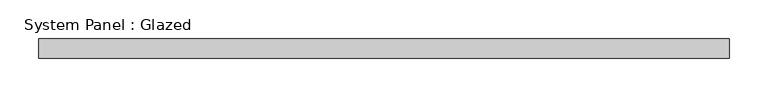
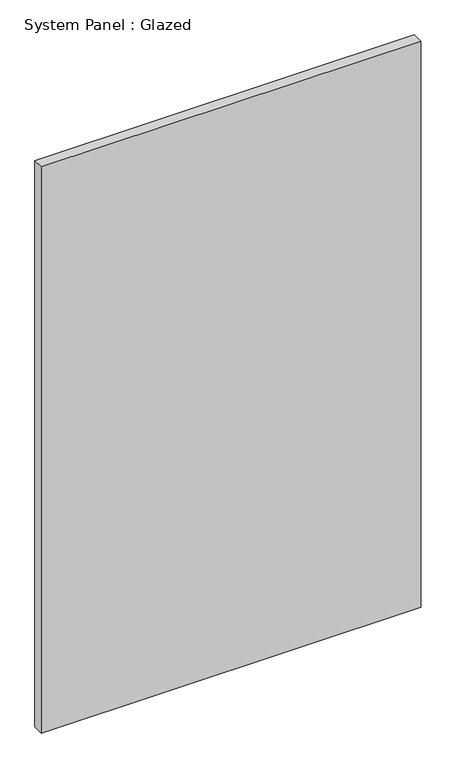
"""IFC4 building model written with IfcOpenShell, lengths in millimetres: plate geometry, System Panel : Glazed."""

from ifc_helpers import new_model, si_unit, origin, origin_with_axes, place, context, project, spatial, polyline, outline, extrude, source, transform, mapped, element, save


def system_panel_glazed_2af6040d(model_context):
    return source(origin(), model_context, "Body", "SweptSolid", [
        extrude(outline(polyline([(447.675, 19.05), (-447.675, 19.05), (-447.675, 44.45), (447.675, 44.45), (447.675, 19.05)])), origin_with_axes(), (0.0, 0.0, 1.0), 1412.658794),
    ])


if __name__ == "__main__":
    model = new_model("IFC4")
    model_context = context("Model", 3, world=origin())
    ifc_project = project(units=[si_unit("LENGTHUNIT", "METRE", prefix="MILLI")], contexts=[model_context])
    site = spatial("IfcSite", under=ifc_project)
    building = spatial("IfcBuilding", under=site)
    placement = place(None, origin())
    system_panel_glazed_shape = system_panel_glazed_2af6040d(model_context)
    element("IfcPlate", 1, ObjectType="System Panel : Glazed", at=placement, inside=building, context=model_context, shape_type="MappedRepresentation", body=[
        mapped(system_panel_glazed_shape, transform((0.0, 0.0, 0.0), x_axis=(1.0, 0.0, 0.0), y_axis=(0.0, 1.0, 0.0), z_axis=(0.0, 0.0, 1.0))),
    ])
    save(model, "model.ifc")

# Revit data of these elements
# Type "System Panel : Glazed"
#   Construction Type Id = "GSP4R"
#   Analytic Construction = "1/8 in Pilkington single glazing"
#   Visual Light Transmittance = 0.9
#   Solar Heat Gain Coefficient = 0.86
#   Heat Transfer Coefficient (U) = 1.18115 BTU/(h·ft²·°F)
#   Define Thermal Properties by = 1
# Element 1 (IfcPlate, "System Panel : Glazed")
#   Materials on its faces: "Glass"
# Materials
#   "Glass": class "Glass", colour RGB 0 128 192, transparency 0.75, Description = "Soda Lime Glass", Cost = 0
